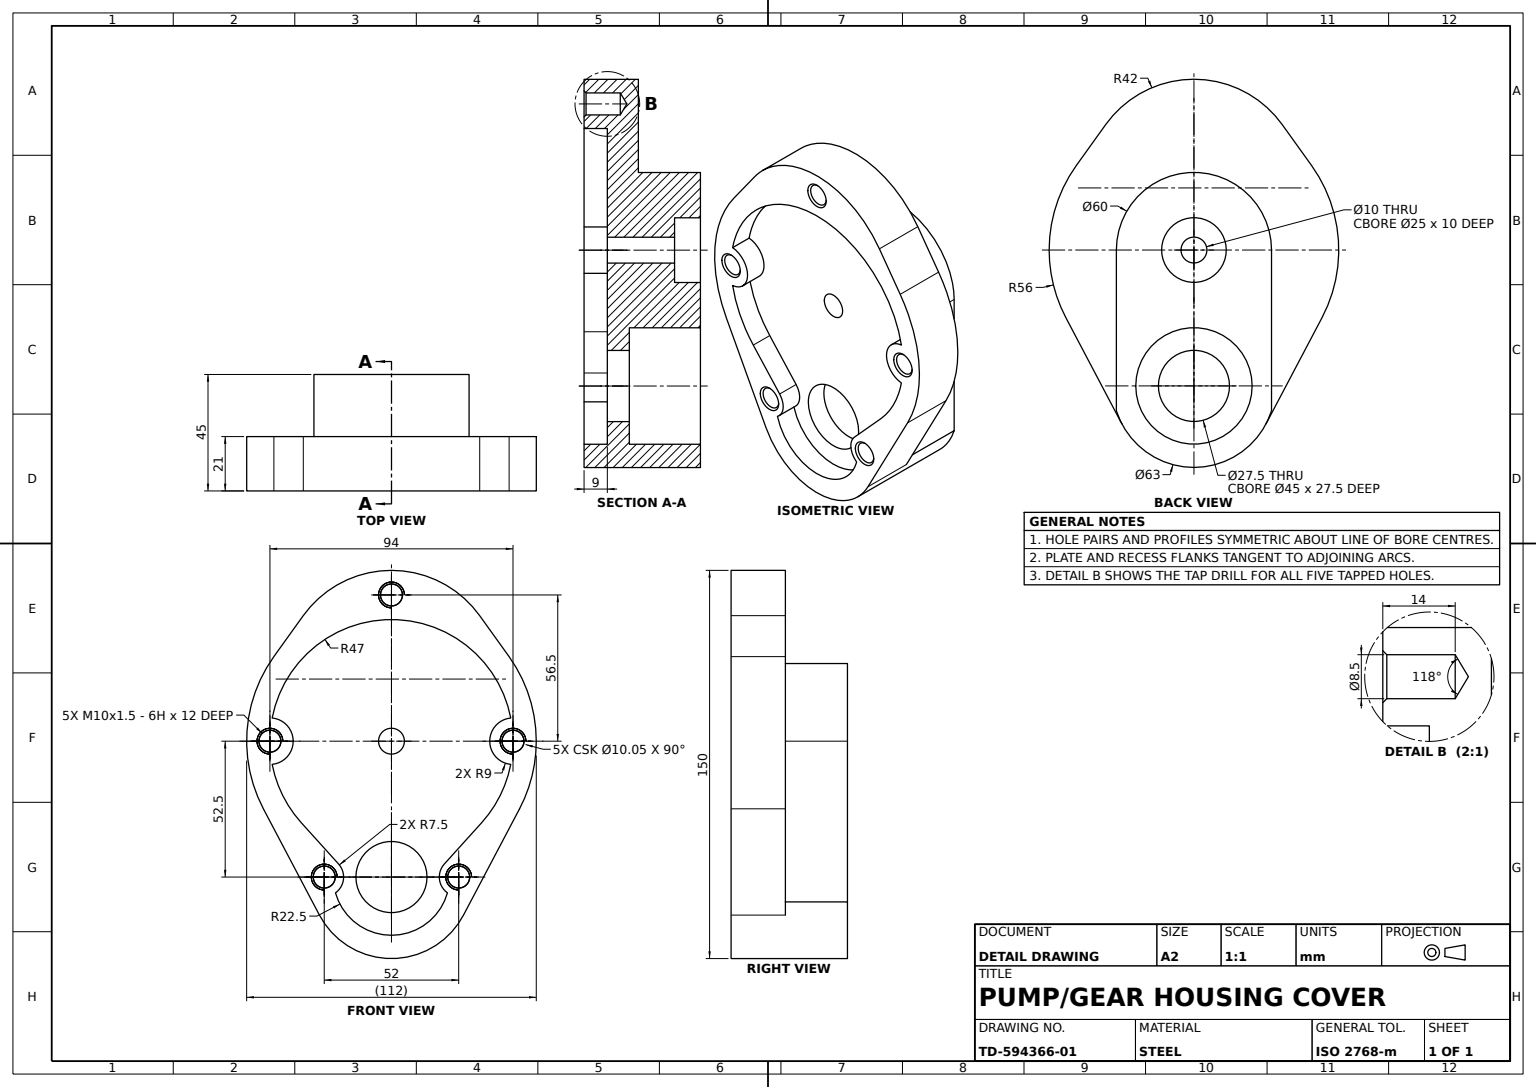
from build123d import *

# Parameters (mm, degrees)
PLATE_PROFILE_SKETCH_W             = 112
PLATE_PROFILE_SKETCH_H             = 150
COVER_PLATE_21MM_DEPTH             = 21
INNER_RECESS_SKETCH_OUTSIDE_W      = 151.674
INNER_RECESS_SKETCH_OUTSIDE_H      = 189.674
INNER_RECESS_CUT_DEPTH             = 21
BORE_BOSS_60_DEPTH                 = 24
FACE_RECESS_9MM_DEPTH              = 9
M10_TAPPED_HOLES_D                 = 8.5
M10_TAPPED_HOLES_DEPTH             = 14
M10_TAPPED_HOLES_CSINK_D           = 10.05
M10_TAPPED_HOLES_CSINK_ANGLE       = 90
M10_TAPPED_HOLES_TIP               = 2.553657631
COUNTERBORED_HOLE_10_D             = 10
COUNTERBORED_HOLE_10_DEPTH         = 100
COUNTERBORED_HOLE_10_CBORE_D       = 25
COUNTERBORED_HOLE_10_CBORE_DEPTH   = 10
COUNTERBORED_BORE_27_5_D           = 27.5
COUNTERBORED_BORE_27_5_DEPTH       = 100
COUNTERBORED_BORE_27_5_CBORE_D     = 45
COUNTERBORED_BORE_27_5_CBORE_DEPTH = 27.5


with BuildPart() as part:
    # Plate Profile Sketch → Cover Plate 21mm (new body)
    with BuildSketch(Plane(origin=(0, 0, 0), x_dir=(0, 0, -1), z_dir=(1, 0, 0))):
        with Locations((0, -9)):
            Rectangle(PLATE_PROFILE_SKETCH_W, PLATE_PROFILE_SKETCH_H)
    extrude(amount=COVER_PLATE_21MM_DEPTH)

    # Inner Recess Sketch outside → Inner Recess Cut (cut)
    with BuildSketch(Plane(origin=(21, 0, 0), x_dir=(0, 0, -1), z_dir=(1, 0, 0))):
        with Locations((0, -9)):
            Rectangle(INNER_RECESS_SKETCH_OUTSIDE_W, INNER_RECESS_SKETCH_OUTSIDE_H)
        with BuildLine():
            Line((-49.528263536, -26.133333333), (-27.859648239, -67.2))
            ThreePointArc((-27.859648239, -67.2), (0, -84), (27.859648239, -67.2))
            Line((27.859648239, -67.2), (49.528263536, -26.133333333))
            ThreePointArc((49.528263536, -26.133333333), (55.868076531, 3.841617458), (45.485040276, 32.666666667))
            Line((45.485040276, 32.666666667), (34.113780207, 48.5))
            ThreePointArc((34.113780207, 48.5), (0, 66), (-34.113780207, 48.5))
            Line((-34.113780207, 48.5), (-45.485040276, 32.666666667))
            ThreePointArc((-45.485040276, 32.666666667), (-55.868076531, 3.841617458), (-49.528263536, -26.133333333))
        make_face(mode=Mode.SUBTRACT)
    extrude(amount=-INNER_RECESS_CUT_DEPTH, mode=Mode.SUBTRACT)

    # Bore Boss Sketch → Bore Boss Ø60 (add)
    with BuildSketch(Plane.ZY):
        with BuildLine():
            Line((30, 0), (30, -62.104686356))
            ThreePointArc((30, -62.104686356), (0, -84), (-30, -62.104686356))
            Line((-30, -62.104686356), (-30, 0))
            ThreePointArc((-30, 0), (0, 30), (30, 0))
        make_face()
    extrude(amount=BORE_BOSS_60_DEPTH)

    # Face Recess Sketch → Face Recess 9mm (cut)
    with BuildSketch(Plane(origin=(21, 0, 0), x_dir=(0, 0, -1), z_dir=(1, 0, 0))):
        with BuildLine():
            Line((-20.437807431, -47.468895368), (-34.856406768, -31.528255696))
            ThreePointArc((-34.856406768, -31.528255696), (-42.040245988, -21.014702408), (-46.138297872, -8.958653328))
            ThreePointArc((-46.138297872, -8.958653328), (-38, 0), (-46.138297872, 8.958653328))
            ThreePointArc((-46.138297872, 8.958653328), (0, 47), (46.138297872, 8.958653328))
            ThreePointArc((46.138297872, 8.958653328), (38, 0), (46.138297872, -8.958653328))
            ThreePointArc((46.138297872, -8.958653328), (42.040245988, -21.014702408), (34.856406768, -31.528255696))
            Line((34.856406768, -31.528255696), (20.437807431, -47.468895368))
            ThreePointArc((20.437807431, -47.468895368), (18.544261668, -53.313612883), (21.653846154, -58.612360162))
            ThreePointArc((21.653846154, -58.612360162), (0, -75), (-21.653846154, -58.612360162))
            ThreePointArc((-21.653846154, -58.612360162), (-18.544261668, -53.313612883), (-20.437807431, -47.468895368))
        make_face()
    extrude(amount=-FACE_RECESS_9MM_DEPTH, mode=Mode.SUBTRACT)

    # M10 Tapped Holes
    with Locations(Plane(origin=(21, 0, 0), x_dir=(0, 0, -1), z_dir=(1, 0, 0))):
        with Locations((-47, 0), (47, 0), (26, -52.5), (-26, -52.5), (0, 56.5)):
            CounterSinkHole(M10_TAPPED_HOLES_D / 2, M10_TAPPED_HOLES_CSINK_D / 2, depth=M10_TAPPED_HOLES_DEPTH, counter_sink_angle=M10_TAPPED_HOLES_CSINK_ANGLE)
            with Locations((0, 0, -(M10_TAPPED_HOLES_DEPTH + M10_TAPPED_HOLES_TIP / 2))):  # 118° drill point
                Cone(0, M10_TAPPED_HOLES_D / 2, M10_TAPPED_HOLES_TIP, mode=Mode.SUBTRACT)

    # Counterbored Hole Ø10
    with Locations(Plane.ZY.offset(24)):
        with Locations((0, 0)):
            CounterBoreHole(COUNTERBORED_HOLE_10_D / 2, COUNTERBORED_HOLE_10_CBORE_D / 2, COUNTERBORED_HOLE_10_CBORE_DEPTH, depth=COUNTERBORED_HOLE_10_DEPTH)

    # Counterbored Bore Ø27.5
    with Locations(Plane.ZY.offset(24)):
        with Locations((0, -52.5)):
            CounterBoreHole(COUNTERBORED_BORE_27_5_D / 2, COUNTERBORED_BORE_27_5_CBORE_D / 2, COUNTERBORED_BORE_27_5_CBORE_DEPTH, depth=COUNTERBORED_BORE_27_5_DEPTH)


solid = part.part
